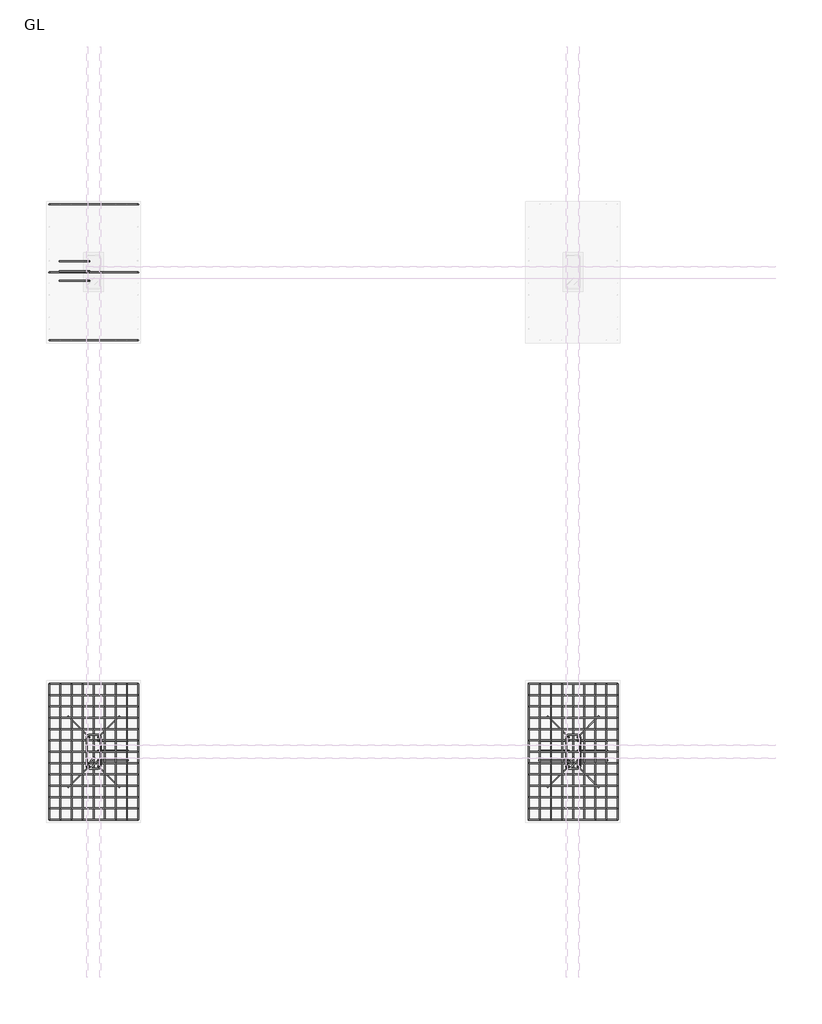
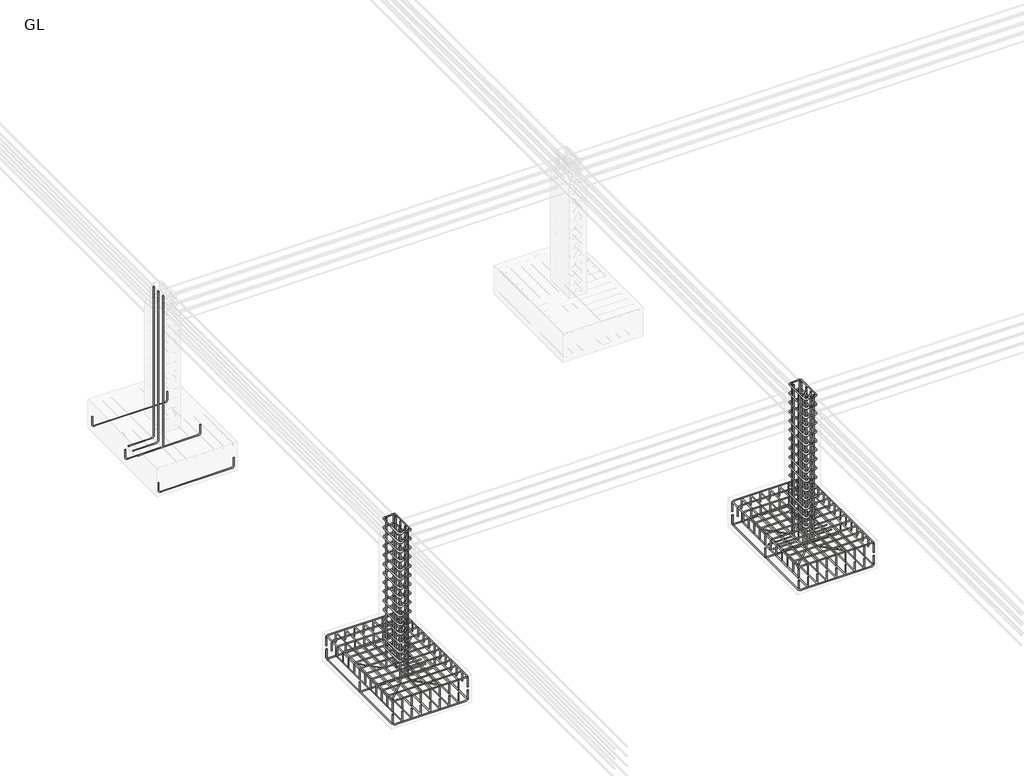
# One storey, part 4 of 16: 23 reinforcing bars.
"""IFC4 building model written with IfcOpenShell, lengths in millimetres."""

from ifc_helpers import new_model, si_unit, point, frame, origin, place, context, project, spatial, polyline, circle_curve, trimmed, segment, composite_curve, source, transform, mapped, element, save
from ifc_brep_helpers import swept_disk

model = new_model("IFC4")

# Units and contexts
model_context = context("Model", 3, world=origin())
ifc_project = project(units=[si_unit("LENGTHUNIT", "METRE", prefix="MILLI")], contexts=[model_context])

# Site, building, storey
site = spatial("IfcSite", under=ifc_project)
building = spatial("IfcBuilding", under=site)
storey = spatial("IfcBuildingStorey", under=building, Name="GL", Elevation=-1829.0)

# Reinforcing bars
placement = place(None, origin())
reinforcing_bar_shape = source(origin(), model_context, "Body", "SolidModel", [
    swept_disk(composite_curve([segment(polyline([(-22242.9544379, -7223.1167521, -2089.0), (-22242.9544379, -7223.1167521, -2213.0)]), True, "CONTINUOUS"), segment(trimmed(circle_curve(frame((-22272.9544379, -7223.1167521, -2213.0), z_axis=(0.0, 1.0, 0.0), x_axis=(30.0, 0.0, 0.0)), 30.0), [point((-22242.9544379, -7223.1167521, -2213.0))], [point((-22272.9544379, -7223.1167521, -2243.0))], True, "CARTESIAN"), True, "CONTINUOUS"), segment(polyline([(-22272.9544379, -7223.1167521, -2243.0), (-23340.9544379, -7223.1167521, -2243.0)]), True, "CONTINUOUS"), segment(trimmed(circle_curve(frame((-23340.9544379, -7223.1167521, -2213.0), z_axis=(0.0, 1.0, 0.0), x_axis=(0.0, 0.0, -30.0)), 30.0), [point((-23340.9544379, -7223.1167521, -2243.0))], [point((-23370.9544379, -7223.1167521, -2213.0))], True, "CARTESIAN"), True, "CONTINUOUS"), segment(polyline([(-23370.9544379, -7223.1167521, -2213.0), (-23370.9544379, -7223.1167521, -2089.0)]), True, "CONTINUOUS")], self_intersect=False), 6.0),
])
element("IfcReinforcingBar", 1, at=placement, inside=storey, context=model_context, shape_type="MappedRepresentation", body=[
    mapped(reinforcing_bar_shape, transform((0.0, 0.0, 0.0), x_axis=(1.0, 0.0, 0.0), y_axis=(0.0, 1.0, 0.0), z_axis=(0.0, 0.0, 1.0))),
    mapped(reinforcing_bar_shape, transform((0.0, -864.0, 0.0), x_axis=(1.0, 0.0, 0.0), y_axis=(0.0, 1.0, 0.0), z_axis=(0.0, 0.0, 1.0))),
    mapped(reinforcing_bar_shape, transform((0.0, -1728.0, 0.0), x_axis=(1.0, 0.0, 0.0), y_axis=(0.0, 1.0, 0.0), z_axis=(0.0, 0.0, 1.0))),
])
reinforcing_bar_2_shape = source(origin(), model_context, "Body", "SolidModel", [
    swept_disk(composite_curve([segment(polyline([(-16146.9544379, -13319.1167521, -2089.0), (-16146.9544379, -13319.1167521, -2213.0)]), True, "CONTINUOUS"), segment(trimmed(circle_curve(frame((-16176.9544379, -13319.1167521, -2213.0), z_axis=(0.0, 1.0, 0.0), x_axis=(30.0, 0.0, 0.0)), 30.0), [point((-16146.9544379, -13319.1167521, -2213.0))], [point((-16176.9544379, -13319.1167521, -2243.0))], True, "CARTESIAN"), True, "CONTINUOUS"), segment(polyline([(-16176.9544379, -13319.1167521, -2243.0), (-17244.9544379, -13319.1167521, -2243.0)]), True, "CONTINUOUS"), segment(trimmed(circle_curve(frame((-17244.9544379, -13319.1167521, -2213.0), z_axis=(0.0, 1.0, 0.0), x_axis=(0.0, 0.0, -30.0)), 30.0), [point((-17244.9544379, -13319.1167521, -2243.0))], [point((-17274.9544379, -13319.1167521, -2213.0))], True, "CARTESIAN"), True, "CONTINUOUS"), segment(polyline([(-17274.9544379, -13319.1167521, -2213.0), (-17274.9544379, -13319.1167521, -2089.0)]), True, "CONTINUOUS")], self_intersect=False), 6.0),
])
element("IfcReinforcingBar", 2, at=placement, inside=storey, context=model_context, shape_type="MappedRepresentation", body=[
    mapped(reinforcing_bar_2_shape, transform((0.0, 0.0, 0.0), x_axis=(1.0, 0.0, 0.0), y_axis=(0.0, 1.0, 0.0), z_axis=(0.0, 0.0, 1.0))),
    mapped(reinforcing_bar_2_shape, transform((0.0, -864.0, 0.0), x_axis=(1.0, 0.0, 0.0), y_axis=(0.0, 1.0, 0.0), z_axis=(0.0, 0.0, 1.0))),
    mapped(reinforcing_bar_2_shape, transform((0.0, -1728.0, 0.0), x_axis=(1.0, 0.0, 0.0), y_axis=(0.0, 1.0, 0.0), z_axis=(0.0, 0.0, 1.0))),
])
reinforcing_bar_3_shape = source(origin(), model_context, "Body", "SolidModel", [
    swept_disk(composite_curve([segment(polyline([(-17274.9544379, -13319.1167521, -2022.436678), (-17274.9544379, -13319.1167521, -1898.436678)]), True, "CONTINUOUS"), segment(trimmed(circle_curve(frame((-17244.9544379, -13319.1167521, -1898.436678), z_axis=(0.0, 1.0, 0.0), x_axis=(-30.0, 0.0, 0.0)), 30.0), [point((-17274.9544379, -13319.1167521, -1898.436678))], [point((-17244.9544379, -13319.1167521, -1868.436678))], True, "CARTESIAN"), True, "CONTINUOUS"), segment(polyline([(-17244.9544379, -13319.1167521, -1868.436678), (-16176.9544379, -13319.1167521, -1868.436678)]), True, "CONTINUOUS"), segment(trimmed(circle_curve(frame((-16176.9544379, -13319.1167521, -1898.436678), z_axis=(0.0, 1.0, 0.0), x_axis=(0.0, 0.0, 30.0)), 30.0), [point((-16176.9544379, -13319.1167521, -1868.436678))], [point((-16146.9544379, -13319.1167521, -1898.436678))], True, "CARTESIAN"), True, "CONTINUOUS"), segment(polyline([(-16146.9544379, -13319.1167521, -1898.436678), (-16146.9544379, -13319.1167521, -2022.436678)]), True, "CONTINUOUS")], self_intersect=False), 6.0),
])
element("IfcReinforcingBar", 3, at=placement, inside=storey, context=model_context, shape_type="MappedRepresentation", body=[
    mapped(reinforcing_bar_3_shape, transform((0.0, 0.0, 0.0), x_axis=(1.0, 0.0, 0.0), y_axis=(0.0, 1.0, 0.0), z_axis=(0.0, 0.0, 1.0))),
    mapped(reinforcing_bar_3_shape, transform((0.0, -144.0, 0.0), x_axis=(1.0, 0.0, 0.0), y_axis=(0.0, 1.0, 0.0), z_axis=(0.0, 0.0, 1.0))),
    mapped(reinforcing_bar_3_shape, transform((0.0, -288.0, 0.0), x_axis=(1.0, 0.0, 0.0), y_axis=(0.0, 1.0, 0.0), z_axis=(0.0, 0.0, 1.0))),
    mapped(reinforcing_bar_3_shape, transform((0.0, -432.0, 0.0), x_axis=(1.0, 0.0, 0.0), y_axis=(0.0, 1.0, 0.0), z_axis=(0.0, 0.0, 1.0))),
    mapped(reinforcing_bar_3_shape, transform((0.0, -576.0, 0.0), x_axis=(1.0, 0.0, 0.0), y_axis=(0.0, 1.0, 0.0), z_axis=(0.0, 0.0, 1.0))),
    mapped(reinforcing_bar_3_shape, transform((0.0, -720.0, 0.0), x_axis=(1.0, 0.0, 0.0), y_axis=(0.0, 1.0, 0.0), z_axis=(0.0, 0.0, 1.0))),
    mapped(reinforcing_bar_3_shape, transform((0.0, -864.0, 0.0), x_axis=(1.0, 0.0, 0.0), y_axis=(0.0, 1.0, 0.0), z_axis=(0.0, 0.0, 1.0))),
    mapped(reinforcing_bar_3_shape, transform((0.0, -1008.0, 0.0), x_axis=(1.0, 0.0, 0.0), y_axis=(0.0, 1.0, 0.0), z_axis=(0.0, 0.0, 1.0))),
    mapped(reinforcing_bar_3_shape, transform((0.0, -1152.0, 0.0), x_axis=(1.0, 0.0, 0.0), y_axis=(0.0, 1.0, 0.0), z_axis=(0.0, 0.0, 1.0))),
    mapped(reinforcing_bar_3_shape, transform((0.0, -1296.0, 0.0), x_axis=(1.0, 0.0, 0.0), y_axis=(0.0, 1.0, 0.0), z_axis=(0.0, 0.0, 1.0))),
    mapped(reinforcing_bar_3_shape, transform((0.0, -1440.0, 0.0), x_axis=(1.0, 0.0, 0.0), y_axis=(0.0, 1.0, 0.0), z_axis=(0.0, 0.0, 1.0))),
    mapped(reinforcing_bar_3_shape, transform((0.0, -1584.0, 0.0), x_axis=(1.0, 0.0, 0.0), y_axis=(0.0, 1.0, 0.0), z_axis=(0.0, 0.0, 1.0))),
    mapped(reinforcing_bar_3_shape, transform((0.0, -1728.0, 0.0), x_axis=(1.0, 0.0, 0.0), y_axis=(0.0, 1.0, 0.0), z_axis=(0.0, 0.0, 1.0))),
])
reinforcing_bar_4_shape = source(origin(), model_context, "Body", "SolidModel", [
    swept_disk(composite_curve([segment(polyline([(-17274.9544379, -15047.1167521, -2027.5081232), (-17274.9544379, -15047.1167521, -1903.5081232)]), True, "CONTINUOUS"), segment(trimmed(circle_curve(frame((-17274.9544379, -15017.1167521, -1903.5081232), z_axis=(-1.0, 0.0, 0.0), x_axis=(0.0, -30.0, 0.0)), 30.0), [point((-17274.9544379, -15047.1167521, -1903.5081232))], [point((-17274.9544379, -15017.1167521, -1873.5081232))], True, "CARTESIAN"), True, "CONTINUOUS"), segment(polyline([(-17274.9544379, -15017.1167521, -1873.5081232), (-17274.9544379, -13349.1167521, -1873.5081232)]), True, "CONTINUOUS"), segment(trimmed(circle_curve(frame((-17274.9544379, -13349.1167521, -1903.5081232), z_axis=(-1.0, 0.0, 0.0), x_axis=(0.0, 0.0, 30.0)), 30.0), [point((-17274.9544379, -13349.1167521, -1873.5081232))], [point((-17274.9544379, -13319.1167521, -1903.5081232))], True, "CARTESIAN"), True, "CONTINUOUS"), segment(polyline([(-17274.9544379, -13319.1167521, -1903.5081232), (-17274.9544379, -13319.1167521, -2027.5081232)]), True, "CONTINUOUS")], self_intersect=False), 6.0),
])
element("IfcReinforcingBar", 4, at=placement, inside=storey, context=model_context, shape_type="MappedRepresentation", body=[
    mapped(reinforcing_bar_4_shape, transform((0.0, 0.0, 0.0), x_axis=(1.0, 0.0, 0.0), y_axis=(0.0, 1.0, 0.0), z_axis=(0.0, 0.0, 1.0))),
    mapped(reinforcing_bar_4_shape, transform((141.0, 0.0, 0.0), x_axis=(1.0, 0.0, 0.0), y_axis=(0.0, 1.0, 0.0), z_axis=(0.0, 0.0, 1.0))),
    mapped(reinforcing_bar_4_shape, transform((282.0, 0.0, 0.0), x_axis=(1.0, 0.0, 0.0), y_axis=(0.0, 1.0, 0.0), z_axis=(0.0, 0.0, 1.0))),
    mapped(reinforcing_bar_4_shape, transform((423.0, 0.0, 0.0), x_axis=(1.0, 0.0, 0.0), y_axis=(0.0, 1.0, 0.0), z_axis=(0.0, 0.0, 1.0))),
    mapped(reinforcing_bar_4_shape, transform((564.0, 0.0, 0.0), x_axis=(1.0, 0.0, 0.0), y_axis=(0.0, 1.0, 0.0), z_axis=(0.0, 0.0, 1.0))),
    mapped(reinforcing_bar_4_shape, transform((705.0, 0.0, 0.0), x_axis=(1.0, 0.0, 0.0), y_axis=(0.0, 1.0, 0.0), z_axis=(0.0, 0.0, 1.0))),
    mapped(reinforcing_bar_4_shape, transform((846.0, 0.0, 0.0), x_axis=(1.0, 0.0, 0.0), y_axis=(0.0, 1.0, 0.0), z_axis=(0.0, 0.0, 1.0))),
    mapped(reinforcing_bar_4_shape, transform((987.0, 0.0, 0.0), x_axis=(1.0, 0.0, 0.0), y_axis=(0.0, 1.0, 0.0), z_axis=(0.0, 0.0, 1.0))),
    mapped(reinforcing_bar_4_shape, transform((1128.0, 0.0, 0.0), x_axis=(1.0, 0.0, 0.0), y_axis=(0.0, 1.0, 0.0), z_axis=(0.0, 0.0, 1.0))),
])
reinforcing_bar_5_shape = source(origin(), model_context, "Body", "SolidModel", [
    swept_disk(composite_curve([segment(polyline([(-16146.9544379, -15047.1167521, -2080.6239909), (-16146.9544379, -15047.1167521, -2204.6239909)]), True, "CONTINUOUS"), segment(trimmed(circle_curve(frame((-16146.9544379, -15017.1167521, -2204.6239909), z_axis=(1.0, 0.0, 0.0), x_axis=(0.0, -30.0, 0.0)), 30.0), [point((-16146.9544379, -15047.1167521, -2204.6239909))], [point((-16146.9544379, -15017.1167521, -2234.6239909))], True, "CARTESIAN"), True, "CONTINUOUS"), segment(polyline([(-16146.9544379, -15017.1167521, -2234.6239909), (-16146.9544379, -13362.1421892, -2234.6239909)]), True, "CONTINUOUS"), segment(trimmed(circle_curve(frame((-16146.9544379, -13362.1421892, -2204.6239909), z_axis=(1.0, 0.0, 0.0), x_axis=(0.0, 0.0, -30.0)), 30.0), [point((-16146.9544379, -13362.1421892, -2234.6239909))], [point((-16146.9544379, -13332.1421892, -2204.6239909))], True, "CARTESIAN"), True, "CONTINUOUS"), segment(polyline([(-16146.9544379, -13332.1421892, -2204.6239909), (-16146.9544379, -13332.1421892, -2080.6239909)]), True, "CONTINUOUS")], self_intersect=False), 6.0),
])
element("IfcReinforcingBar", 5, at=placement, inside=storey, context=model_context, shape_type="MappedRepresentation", body=[
    mapped(reinforcing_bar_5_shape, transform((0.0, 0.0, 0.0), x_axis=(1.0, 0.0, 0.0), y_axis=(0.0, 1.0, 0.0), z_axis=(0.0, 0.0, 1.0))),
    mapped(reinforcing_bar_5_shape, transform((-141.0, 0.0, 0.0), x_axis=(1.0, 0.0, 0.0), y_axis=(0.0, 1.0, 0.0), z_axis=(0.0, 0.0, 1.0))),
    mapped(reinforcing_bar_5_shape, transform((-282.0, 0.0, 0.0), x_axis=(1.0, 0.0, 0.0), y_axis=(0.0, 1.0, 0.0), z_axis=(0.0, 0.0, 1.0))),
    mapped(reinforcing_bar_5_shape, transform((-423.0, 0.0, 0.0), x_axis=(1.0, 0.0, 0.0), y_axis=(0.0, 1.0, 0.0), z_axis=(0.0, 0.0, 1.0))),
    mapped(reinforcing_bar_5_shape, transform((-564.0, 0.0, 0.0), x_axis=(1.0, 0.0, 0.0), y_axis=(0.0, 1.0, 0.0), z_axis=(0.0, 0.0, 1.0))),
    mapped(reinforcing_bar_5_shape, transform((-705.0, 0.0, 0.0), x_axis=(1.0, 0.0, 0.0), y_axis=(0.0, 1.0, 0.0), z_axis=(0.0, 0.0, 1.0))),
    mapped(reinforcing_bar_5_shape, transform((-846.0, 0.0, 0.0), x_axis=(1.0, 0.0, 0.0), y_axis=(0.0, 1.0, 0.0), z_axis=(0.0, 0.0, 1.0))),
    mapped(reinforcing_bar_5_shape, transform((-987.0, 0.0, 0.0), x_axis=(1.0, 0.0, 0.0), y_axis=(0.0, 1.0, 0.0), z_axis=(0.0, 0.0, 1.0))),
    mapped(reinforcing_bar_5_shape, transform((-1128.0, 0.0, 0.0), x_axis=(1.0, 0.0, 0.0), y_axis=(0.0, 1.0, 0.0), z_axis=(0.0, 0.0, 1.0))),
])
reinforcing_bar_6_shape = source(origin(), model_context, "Body", "SolidModel", [
    swept_disk(composite_curve([segment(polyline([(-22242.9544379, -13319.1167521, -2089.0), (-22242.9544379, -13319.1167521, -2213.0)]), True, "CONTINUOUS"), segment(trimmed(circle_curve(frame((-22272.9544379, -13319.1167521, -2213.0), z_axis=(0.0, 1.0, 0.0), x_axis=(30.0, 0.0, 0.0)), 30.0), [point((-22242.9544379, -13319.1167521, -2213.0))], [point((-22272.9544379, -13319.1167521, -2243.0))], True, "CARTESIAN"), True, "CONTINUOUS"), segment(polyline([(-22272.9544379, -13319.1167521, -2243.0), (-23340.9544379, -13319.1167521, -2243.0)]), True, "CONTINUOUS"), segment(trimmed(circle_curve(frame((-23340.9544379, -13319.1167521, -2213.0), z_axis=(0.0, 1.0, 0.0), x_axis=(0.0, 0.0, -30.0)), 30.0), [point((-23340.9544379, -13319.1167521, -2243.0))], [point((-23370.9544379, -13319.1167521, -2213.0))], True, "CARTESIAN"), True, "CONTINUOUS"), segment(polyline([(-23370.9544379, -13319.1167521, -2213.0), (-23370.9544379, -13319.1167521, -2089.0)]), True, "CONTINUOUS")], self_intersect=False), 6.0),
])
element("IfcReinforcingBar", 6, at=placement, inside=storey, context=model_context, shape_type="MappedRepresentation", body=[
    mapped(reinforcing_bar_6_shape, transform((0.0, 0.0, 0.0), x_axis=(1.0, 0.0, 0.0), y_axis=(0.0, 1.0, 0.0), z_axis=(0.0, 0.0, 1.0))),
    mapped(reinforcing_bar_6_shape, transform((0.0, -864.0, 0.0), x_axis=(1.0, 0.0, 0.0), y_axis=(0.0, 1.0, 0.0), z_axis=(0.0, 0.0, 1.0))),
    mapped(reinforcing_bar_6_shape, transform((0.0, -1728.0, 0.0), x_axis=(1.0, 0.0, 0.0), y_axis=(0.0, 1.0, 0.0), z_axis=(0.0, 0.0, 1.0))),
])
reinforcing_bar_7_shape = source(origin(), model_context, "Body", "SolidModel", [
    swept_disk(composite_curve([segment(polyline([(-23370.9544379, -13319.1167521, -2022.436678), (-23370.9544379, -13319.1167521, -1898.436678)]), True, "CONTINUOUS"), segment(trimmed(circle_curve(frame((-23340.9544379, -13319.1167521, -1898.436678), z_axis=(0.0, 1.0, 0.0), x_axis=(-30.0, 0.0, 0.0)), 30.0), [point((-23370.9544379, -13319.1167521, -1898.436678))], [point((-23340.9544379, -13319.1167521, -1868.436678))], True, "CARTESIAN"), True, "CONTINUOUS"), segment(polyline([(-23340.9544379, -13319.1167521, -1868.436678), (-22272.9544379, -13319.1167521, -1868.436678)]), True, "CONTINUOUS"), segment(trimmed(circle_curve(frame((-22272.9544379, -13319.1167521, -1898.436678), z_axis=(0.0, 1.0, 0.0), x_axis=(0.0, 0.0, 30.0)), 30.0), [point((-22272.9544379, -13319.1167521, -1868.436678))], [point((-22242.9544379, -13319.1167521, -1898.436678))], True, "CARTESIAN"), True, "CONTINUOUS"), segment(polyline([(-22242.9544379, -13319.1167521, -1898.436678), (-22242.9544379, -13319.1167521, -2022.436678)]), True, "CONTINUOUS")], self_intersect=False), 6.0),
])
element("IfcReinforcingBar", 7, at=placement, inside=storey, context=model_context, shape_type="MappedRepresentation", body=[
    mapped(reinforcing_bar_7_shape, transform((0.0, 0.0, 0.0), x_axis=(1.0, 0.0, 0.0), y_axis=(0.0, 1.0, 0.0), z_axis=(0.0, 0.0, 1.0))),
    mapped(reinforcing_bar_7_shape, transform((0.0, -144.0, 0.0), x_axis=(1.0, 0.0, 0.0), y_axis=(0.0, 1.0, 0.0), z_axis=(0.0, 0.0, 1.0))),
    mapped(reinforcing_bar_7_shape, transform((0.0, -288.0, 0.0), x_axis=(1.0, 0.0, 0.0), y_axis=(0.0, 1.0, 0.0), z_axis=(0.0, 0.0, 1.0))),
    mapped(reinforcing_bar_7_shape, transform((0.0, -432.0, 0.0), x_axis=(1.0, 0.0, 0.0), y_axis=(0.0, 1.0, 0.0), z_axis=(0.0, 0.0, 1.0))),
    mapped(reinforcing_bar_7_shape, transform((0.0, -576.0, 0.0), x_axis=(1.0, 0.0, 0.0), y_axis=(0.0, 1.0, 0.0), z_axis=(0.0, 0.0, 1.0))),
    mapped(reinforcing_bar_7_shape, transform((0.0, -720.0, 0.0), x_axis=(1.0, 0.0, 0.0), y_axis=(0.0, 1.0, 0.0), z_axis=(0.0, 0.0, 1.0))),
    mapped(reinforcing_bar_7_shape, transform((0.0, -864.0, 0.0), x_axis=(1.0, 0.0, 0.0), y_axis=(0.0, 1.0, 0.0), z_axis=(0.0, 0.0, 1.0))),
    mapped(reinforcing_bar_7_shape, transform((0.0, -1008.0, 0.0), x_axis=(1.0, 0.0, 0.0), y_axis=(0.0, 1.0, 0.0), z_axis=(0.0, 0.0, 1.0))),
    mapped(reinforcing_bar_7_shape, transform((0.0, -1152.0, 0.0), x_axis=(1.0, 0.0, 0.0), y_axis=(0.0, 1.0, 0.0), z_axis=(0.0, 0.0, 1.0))),
    mapped(reinforcing_bar_7_shape, transform((0.0, -1296.0, 0.0), x_axis=(1.0, 0.0, 0.0), y_axis=(0.0, 1.0, 0.0), z_axis=(0.0, 0.0, 1.0))),
    mapped(reinforcing_bar_7_shape, transform((0.0, -1440.0, 0.0), x_axis=(1.0, 0.0, 0.0), y_axis=(0.0, 1.0, 0.0), z_axis=(0.0, 0.0, 1.0))),
    mapped(reinforcing_bar_7_shape, transform((0.0, -1584.0, 0.0), x_axis=(1.0, 0.0, 0.0), y_axis=(0.0, 1.0, 0.0), z_axis=(0.0, 0.0, 1.0))),
    mapped(reinforcing_bar_7_shape, transform((0.0, -1728.0, 0.0), x_axis=(1.0, 0.0, 0.0), y_axis=(0.0, 1.0, 0.0), z_axis=(0.0, 0.0, 1.0))),
])
reinforcing_bar_8_shape = source(origin(), model_context, "Body", "SolidModel", [
    swept_disk(composite_curve([segment(polyline([(-23370.9544379, -15047.1167521, -2027.5081232), (-23370.9544379, -15047.1167521, -1903.5081232)]), True, "CONTINUOUS"), segment(trimmed(circle_curve(frame((-23370.9544379, -15017.1167521, -1903.5081232), z_axis=(-1.0, 0.0, 0.0), x_axis=(0.0, -30.0, 0.0)), 30.0), [point((-23370.9544379, -15047.1167521, -1903.5081232))], [point((-23370.9544379, -15017.1167521, -1873.5081232))], True, "CARTESIAN"), True, "CONTINUOUS"), segment(polyline([(-23370.9544379, -15017.1167521, -1873.5081232), (-23370.9544379, -13349.1167521, -1873.5081232)]), True, "CONTINUOUS"), segment(trimmed(circle_curve(frame((-23370.9544379, -13349.1167521, -1903.5081232), z_axis=(-1.0, 0.0, 0.0), x_axis=(0.0, 0.0, 30.0)), 30.0), [point((-23370.9544379, -13349.1167521, -1873.5081232))], [point((-23370.9544379, -13319.1167521, -1903.5081232))], True, "CARTESIAN"), True, "CONTINUOUS"), segment(polyline([(-23370.9544379, -13319.1167521, -1903.5081232), (-23370.9544379, -13319.1167521, -2027.5081232)]), True, "CONTINUOUS")], self_intersect=False), 6.0),
])
element("IfcReinforcingBar", 8, at=placement, inside=storey, context=model_context, shape_type="MappedRepresentation", body=[
    mapped(reinforcing_bar_8_shape, transform((0.0, 0.0, 0.0), x_axis=(1.0, 0.0, 0.0), y_axis=(0.0, 1.0, 0.0), z_axis=(0.0, 0.0, 1.0))),
    mapped(reinforcing_bar_8_shape, transform((141.0, 0.0, 0.0), x_axis=(1.0, 0.0, 0.0), y_axis=(0.0, 1.0, 0.0), z_axis=(0.0, 0.0, 1.0))),
    mapped(reinforcing_bar_8_shape, transform((282.0, 0.0, 0.0), x_axis=(1.0, 0.0, 0.0), y_axis=(0.0, 1.0, 0.0), z_axis=(0.0, 0.0, 1.0))),
    mapped(reinforcing_bar_8_shape, transform((423.0, 0.0, 0.0), x_axis=(1.0, 0.0, 0.0), y_axis=(0.0, 1.0, 0.0), z_axis=(0.0, 0.0, 1.0))),
    mapped(reinforcing_bar_8_shape, transform((564.0, 0.0, 0.0), x_axis=(1.0, 0.0, 0.0), y_axis=(0.0, 1.0, 0.0), z_axis=(0.0, 0.0, 1.0))),
    mapped(reinforcing_bar_8_shape, transform((705.0, 0.0, 0.0), x_axis=(1.0, 0.0, 0.0), y_axis=(0.0, 1.0, 0.0), z_axis=(0.0, 0.0, 1.0))),
    mapped(reinforcing_bar_8_shape, transform((846.0, 0.0, 0.0), x_axis=(1.0, 0.0, 0.0), y_axis=(0.0, 1.0, 0.0), z_axis=(0.0, 0.0, 1.0))),
    mapped(reinforcing_bar_8_shape, transform((987.0, 0.0, 0.0), x_axis=(1.0, 0.0, 0.0), y_axis=(0.0, 1.0, 0.0), z_axis=(0.0, 0.0, 1.0))),
    mapped(reinforcing_bar_8_shape, transform((1128.0, 0.0, 0.0), x_axis=(1.0, 0.0, 0.0), y_axis=(0.0, 1.0, 0.0), z_axis=(0.0, 0.0, 1.0))),
])
reinforcing_bar_9_shape = source(origin(), model_context, "Body", "SolidModel", [
    swept_disk(composite_curve([segment(polyline([(-22242.9544379, -15047.1167521, -2080.6239909), (-22242.9544379, -15047.1167521, -2204.6239909)]), True, "CONTINUOUS"), segment(trimmed(circle_curve(frame((-22242.9544379, -15017.1167521, -2204.6239909), z_axis=(1.0, 0.0, 0.0), x_axis=(0.0, -30.0, 0.0)), 30.0), [point((-22242.9544379, -15047.1167521, -2204.6239909))], [point((-22242.9544379, -15017.1167521, -2234.6239909))], True, "CARTESIAN"), True, "CONTINUOUS"), segment(polyline([(-22242.9544379, -15017.1167521, -2234.6239909), (-22242.9544379, -13362.1421892, -2234.6239909)]), True, "CONTINUOUS"), segment(trimmed(circle_curve(frame((-22242.9544379, -13362.1421892, -2204.6239909), z_axis=(1.0, 0.0, 0.0), x_axis=(0.0, 0.0, -30.0)), 30.0), [point((-22242.9544379, -13362.1421892, -2234.6239909))], [point((-22242.9544379, -13332.1421892, -2204.6239909))], True, "CARTESIAN"), True, "CONTINUOUS"), segment(polyline([(-22242.9544379, -13332.1421892, -2204.6239909), (-22242.9544379, -13332.1421892, -2080.6239909)]), True, "CONTINUOUS")], self_intersect=False), 6.0),
])
element("IfcReinforcingBar", 9, at=placement, inside=storey, context=model_context, shape_type="MappedRepresentation", body=[
    mapped(reinforcing_bar_9_shape, transform((0.0, 0.0, 0.0), x_axis=(1.0, 0.0, 0.0), y_axis=(0.0, 1.0, 0.0), z_axis=(0.0, 0.0, 1.0))),
    mapped(reinforcing_bar_9_shape, transform((-141.0, 0.0, 0.0), x_axis=(1.0, 0.0, 0.0), y_axis=(0.0, 1.0, 0.0), z_axis=(0.0, 0.0, 1.0))),
    mapped(reinforcing_bar_9_shape, transform((-282.0, 0.0, 0.0), x_axis=(1.0, 0.0, 0.0), y_axis=(0.0, 1.0, 0.0), z_axis=(0.0, 0.0, 1.0))),
    mapped(reinforcing_bar_9_shape, transform((-423.0, 0.0, 0.0), x_axis=(1.0, 0.0, 0.0), y_axis=(0.0, 1.0, 0.0), z_axis=(0.0, 0.0, 1.0))),
    mapped(reinforcing_bar_9_shape, transform((-564.0, 0.0, 0.0), x_axis=(1.0, 0.0, 0.0), y_axis=(0.0, 1.0, 0.0), z_axis=(0.0, 0.0, 1.0))),
    mapped(reinforcing_bar_9_shape, transform((-705.0, 0.0, 0.0), x_axis=(1.0, 0.0, 0.0), y_axis=(0.0, 1.0, 0.0), z_axis=(0.0, 0.0, 1.0))),
    mapped(reinforcing_bar_9_shape, transform((-846.0, 0.0, 0.0), x_axis=(1.0, 0.0, 0.0), y_axis=(0.0, 1.0, 0.0), z_axis=(0.0, 0.0, 1.0))),
    mapped(reinforcing_bar_9_shape, transform((-987.0, 0.0, 0.0), x_axis=(1.0, 0.0, 0.0), y_axis=(0.0, 1.0, 0.0), z_axis=(0.0, 0.0, 1.0))),
    mapped(reinforcing_bar_9_shape, transform((-1128.0, 0.0, 0.0), x_axis=(1.0, 0.0, 0.0), y_axis=(0.0, 1.0, 0.0), z_axis=(0.0, 0.0, 1.0))),
])
reinforcing_bar_10_shape = source(origin(), model_context, "Body", "SolidModel", [
    swept_disk(composite_curve([segment(polyline([(-22864.0642232, -8194.9117405, 241.0), (-22864.0642232, -8194.9117405, -2129.0)]), True, "CONTINUOUS"), segment(trimmed(circle_curve(frame((-22894.0642232, -8194.9117405, -2129.0), z_axis=(0.0, 1.0, 0.0), x_axis=(30.0, 0.0, 0.0)), 30.0), [point((-22864.0642232, -8194.9117405, -2129.0))], [point((-22894.0642232, -8194.9117405, -2159.0))], True, "CARTESIAN"), True, "CONTINUOUS"), segment(polyline([(-22894.0642232, -8194.9117405, -2159.0), (-23244.0642232, -8194.9117405, -2159.0)]), True, "CONTINUOUS")], self_intersect=False), 6.0),
])
element("IfcReinforcingBar", 10, at=placement, inside=storey, context=model_context, shape_type="MappedRepresentation", body=[
    mapped(reinforcing_bar_10_shape, transform((0.0, 0.0, 0.0), x_axis=(1.0, 0.0, 0.0), y_axis=(0.0, 1.0, 0.0), z_axis=(0.0, 0.0, 1.0))),
    mapped(reinforcing_bar_10_shape, transform((0.0, 123.5823926, 0.0), x_axis=(1.0, 0.0, 0.0), y_axis=(0.0, 1.0, 0.0), z_axis=(0.0, 0.0, 1.0))),
    mapped(reinforcing_bar_10_shape, transform((0.0, 247.1647853, 0.0), x_axis=(1.0, 0.0, 0.0), y_axis=(0.0, 1.0, 0.0), z_axis=(0.0, 0.0, 1.0))),
])
reinforcing_bar_11_shape = source(origin(), model_context, "Body", "SolidModel", [
    swept_disk(composite_curve([segment(polyline([(-22799.4864005, -14258.2223078, -1793.0), (-22887.1676414, -14345.9035486, -1793.0)]), True, "CONTINUOUS"), segment(trimmed(circle_curve(frame((-22865.9544379, -14367.1167521, -1793.0), z_axis=(0.0, 0.0, 1.0), x_axis=(-21.21320349999951, 21.213203500001327, 0.0)), 30.0), [point((-22887.1676414, -14345.9035486, -1793.0))], [point((-22865.9544379, -14397.1167521, -1793.0))], True, "CARTESIAN"), True, "CONTINUOUS"), segment(polyline([(-22865.9544379, -14397.1167521, -1793.0), (-22747.9544379, -14397.1167521, -1793.0)]), True, "CONTINUOUS"), segment(trimmed(circle_curve(frame((-22747.9544379, -14367.1167521, -1793.0), z_axis=(0.0, 0.0, 1.0), x_axis=(0.0, -30.0, 0.0)), 30.0), [point((-22747.9544379, -14397.1167521, -1793.0))], [point((-22717.9544379, -14367.1167521, -1793.0))], True, "CARTESIAN"), True, "CONTINUOUS"), segment(polyline([(-22717.9544379, -14367.1167521, -1793.0), (-22717.9544379, -13999.1167521, -1793.0)]), True, "CONTINUOUS"), segment(trimmed(circle_curve(frame((-22747.8864962, -13999.1167521, -1795.0178916), z_axis=(-0.06726305234213417, 0.0, 0.9977352764083365), x_axis=(29.93205830000079, 0.0, 2.0178915999999845)), 30.0), [point((-22717.9544379, -13999.1167521, -1793.0))], [point((-22747.8864962, -13969.1167521, -1795.0178916))], True, "CARTESIAN"), True, "CONTINUOUS"), segment(polyline([(-22747.8864962, -13969.1167521, -1795.0178916), (-22866.0223796, -13969.1167521, -1802.9821084)]), True, "CONTINUOUS"), segment(trimmed(circle_curve(frame((-22866.0223796, -13999.1167521, -1802.9821084), z_axis=(-0.06726305234213417, 0.0, 0.9977352764083365), x_axis=(0.0, 30.0, 0.0)), 30.0), [point((-22866.0223796, -13969.1167521, -1802.9821084))], [point((-22895.9544379, -13999.1167521, -1805.0))], True, "CARTESIAN"), True, "CONTINUOUS"), segment(polyline([(-22895.9544379, -13999.1167521, -1805.0), (-22895.9544379, -14367.1167521, -1805.0)]), True, "CONTINUOUS"), segment(trimmed(circle_curve(frame((-22865.9544379, -14367.1167521, -1805.0), z_axis=(0.0, 0.0, 1.0), x_axis=(-30.0, 0.0, 0.0)), 30.0), [point((-22895.9544379, -14367.1167521, -1805.0))], [point((-22844.7412345, -14388.3299555, -1805.0))], True, "CARTESIAN"), True, "CONTINUOUS"), segment(polyline([(-22844.7412345, -14388.3299555, -1805.0), (-22757.0599936, -14300.6487146, -1805.0)]), True, "CONTINUOUS")], self_intersect=False), 6.0),
])
element("IfcReinforcingBar", 11, at=placement, inside=storey, context=model_context, shape_type="MappedRepresentation", body=[
    mapped(reinforcing_bar_11_shape, transform((0.0, 0.0, 0.0), x_axis=(1.0, 0.0, 0.0), y_axis=(0.0, 1.0, 0.0), z_axis=(0.0, 0.0, 1.0))),
    mapped(reinforcing_bar_11_shape, transform((0.0, 0.0, 144.8571429), x_axis=(1.0, 0.0, 0.0), y_axis=(0.0, 1.0, 0.0), z_axis=(0.0, 0.0, 1.0))),
    mapped(reinforcing_bar_11_shape, transform((0.0, 0.0, 289.7142857), x_axis=(1.0, 0.0, 0.0), y_axis=(0.0, 1.0, 0.0), z_axis=(0.0, 0.0, 1.0))),
    mapped(reinforcing_bar_11_shape, transform((0.0, 0.0, 434.5714286), x_axis=(1.0, 0.0, 0.0), y_axis=(0.0, 1.0, 0.0), z_axis=(0.0, 0.0, 1.0))),
    mapped(reinforcing_bar_11_shape, transform((0.0, 0.0, 579.4285714), x_axis=(1.0, 0.0, 0.0), y_axis=(0.0, 1.0, 0.0), z_axis=(0.0, 0.0, 1.0))),
    mapped(reinforcing_bar_11_shape, transform((0.0, 0.0, 724.2857143), x_axis=(1.0, 0.0, 0.0), y_axis=(0.0, 1.0, 0.0), z_axis=(0.0, 0.0, 1.0))),
    mapped(reinforcing_bar_11_shape, transform((0.0, 0.0, 869.1428571), x_axis=(1.0, 0.0, 0.0), y_axis=(0.0, 1.0, 0.0), z_axis=(0.0, 0.0, 1.0))),
    mapped(reinforcing_bar_11_shape, transform((0.0, 0.0, 1014.0), x_axis=(1.0, 0.0, 0.0), y_axis=(0.0, 1.0, 0.0), z_axis=(0.0, 0.0, 1.0))),
    mapped(reinforcing_bar_11_shape, transform((0.0, 0.0, 1158.8571429), x_axis=(1.0, 0.0, 0.0), y_axis=(0.0, 1.0, 0.0), z_axis=(0.0, 0.0, 1.0))),
    mapped(reinforcing_bar_11_shape, transform((0.0, 0.0, 1303.7142857), x_axis=(1.0, 0.0, 0.0), y_axis=(0.0, 1.0, 0.0), z_axis=(0.0, 0.0, 1.0))),
    mapped(reinforcing_bar_11_shape, transform((0.0, 0.0, 1448.5714286), x_axis=(1.0, 0.0, 0.0), y_axis=(0.0, 1.0, 0.0), z_axis=(0.0, 0.0, 1.0))),
    mapped(reinforcing_bar_11_shape, transform((0.0, 0.0, 1593.4285714), x_axis=(1.0, 0.0, 0.0), y_axis=(0.0, 1.0, 0.0), z_axis=(0.0, 0.0, 1.0))),
    mapped(reinforcing_bar_11_shape, transform((0.0, 0.0, 1738.2857143), x_axis=(1.0, 0.0, 0.0), y_axis=(0.0, 1.0, 0.0), z_axis=(0.0, 0.0, 1.0))),
    mapped(reinforcing_bar_11_shape, transform((0.0, 0.0, 1883.1428571), x_axis=(1.0, 0.0, 0.0), y_axis=(0.0, 1.0, 0.0), z_axis=(0.0, 0.0, 1.0))),
    mapped(reinforcing_bar_11_shape, transform((0.0, 0.0, 2028.0), x_axis=(1.0, 0.0, 0.0), y_axis=(0.0, 1.0, 0.0), z_axis=(0.0, 0.0, 1.0))),
])
element("IfcReinforcingBar", 12, at=placement, inside=storey, context=model_context, shape_type="SolidModel", body=[
    swept_disk(composite_curve([segment(polyline([(-22864.0642232, -14368.0642439, 241.0), (-22864.0642232, -14368.0642439, -2129.0)]), True, "CONTINUOUS"), segment(trimmed(circle_curve(frame((-22885.2774266, -14389.2774473, -2129.0), z_axis=(-0.7071067811865187, 0.7071067811865764, 0.0), x_axis=(21.213203400002385, 21.213203400000566, 0.0)), 30.0), [point((-22864.0642232, -14368.0642439, -2129.0))], [point((-22885.2774266, -14389.2774473, -2159.0))], True, "CARTESIAN"), True, "CONTINUOUS"), segment(polyline([(-22885.2774266, -14389.2774473, -2159.0), (-23132.7648, -14636.7648207, -2159.0)]), True, "CONTINUOUS")], self_intersect=False), 6.0),
])
element("IfcReinforcingBar", 13, at=placement, inside=storey, context=model_context, shape_type="SolidModel", body=[
    swept_disk(composite_curve([segment(polyline([(-22864.0642232, -13998.1692603, 241.0), (-22864.0642232, -13998.1692603, -2129.0)]), True, "CONTINUOUS"), segment(trimmed(circle_curve(frame((-22885.2774266, -13976.9560568, -2129.0), z_axis=(0.7071067811865218, 0.7071067811865733, 0.0), x_axis=(21.213203400002385, -21.21320349999951, 0.0)), 30.0), [point((-22864.0642232, -13998.1692603, -2129.0))], [point((-22885.2774266, -13976.9560568, -2159.0))], True, "CARTESIAN"), True, "CONTINUOUS"), segment(polyline([(-22885.2774266, -13976.9560568, -2159.0), (-23132.7648, -13729.4686834, -2159.0)]), True, "CONTINUOUS")], self_intersect=False), 6.0),
])
element("IfcReinforcingBar", 14, at=placement, inside=storey, context=model_context, shape_type="SolidModel", body=[
    swept_disk(composite_curve([segment(polyline([(-22749.8446527, -14368.0642439, 241.0), (-22749.8446527, -14368.0642439, -2129.0)]), True, "CONTINUOUS"), segment(trimmed(circle_curve(frame((-22728.6314492, -14389.2774473, -2129.0), z_axis=(-0.7071067811865248, -0.7071067811865703, 0.0), x_axis=(-21.213203500003146, 21.213203400000566, 0.0)), 30.0), [point((-22749.8446527, -14368.0642439, -2129.0))], [point((-22728.6314492, -14389.2774473, -2159.0))], True, "CARTESIAN"), True, "CONTINUOUS"), segment(polyline([(-22728.6314492, -14389.2774473, -2159.0), (-22481.1440758, -14636.7648207, -2159.0)]), True, "CONTINUOUS")], self_intersect=False), 6.0),
])
element("IfcReinforcingBar", 15, at=placement, inside=storey, context=model_context, shape_type="SolidModel", body=[
    swept_disk(composite_curve([segment(polyline([(-22749.8446527, -13998.1692603, 241.0), (-22749.8446527, -13998.1692603, -2129.0)]), True, "CONTINUOUS"), segment(trimmed(circle_curve(frame((-22728.6314492, -13976.9560568, -2129.0), z_axis=(0.7071067811865157, -0.7071067811865794, 0.0), x_axis=(-21.213203500003146, -21.21320349999951, 0.0)), 30.0), [point((-22749.8446527, -13998.1692603, -2129.0))], [point((-22728.6314492, -13976.9560568, -2159.0))], True, "CARTESIAN"), True, "CONTINUOUS"), segment(polyline([(-22728.6314492, -13976.9560568, -2159.0), (-22481.1440758, -13729.4686834, -2159.0)]), True, "CONTINUOUS")], self_intersect=False), 6.0),
])
reinforcing_bar_12_shape = source(origin(), model_context, "Body", "SolidModel", [
    swept_disk(composite_curve([segment(polyline([(-22749.8446527, -14290.9117405, 241.0), (-22749.8446527, -14290.9117405, -2129.0)]), True, "CONTINUOUS"), segment(trimmed(circle_curve(frame((-22719.8446527, -14290.9117405, -2129.0), z_axis=(0.0, -1.0, 0.0), x_axis=(-30.0, 0.0, 0.0)), 30.0), [point((-22749.8446527, -14290.9117405, -2129.0))], [point((-22719.8446527, -14290.9117405, -2159.0))], True, "CARTESIAN"), True, "CONTINUOUS"), segment(polyline([(-22719.8446527, -14290.9117405, -2159.0), (-22369.8446527, -14290.9117405, -2159.0)]), True, "CONTINUOUS")], self_intersect=False), 6.0),
])
element("IfcReinforcingBar", 16, at=placement, inside=storey, context=model_context, shape_type="MappedRepresentation", body=[
    mapped(reinforcing_bar_12_shape, transform((0.0, 0.0, 0.0), x_axis=(1.0, 0.0, 0.0), y_axis=(0.0, 1.0, 0.0), z_axis=(0.0, 0.0, 1.0))),
    mapped(reinforcing_bar_12_shape, transform((0.0, 123.5823926, 0.0), x_axis=(1.0, 0.0, 0.0), y_axis=(0.0, 1.0, 0.0), z_axis=(0.0, 0.0, 1.0))),
    mapped(reinforcing_bar_12_shape, transform((0.0, 247.1647853, 0.0), x_axis=(1.0, 0.0, 0.0), y_axis=(0.0, 1.0, 0.0), z_axis=(0.0, 0.0, 1.0))),
])
reinforcing_bar_13_shape = source(origin(), model_context, "Body", "SolidModel", [
    swept_disk(composite_curve([segment(polyline([(-16703.4864005, -14258.2223078, -1793.0), (-16791.1676414, -14345.9035486, -1793.0)]), True, "CONTINUOUS"), segment(trimmed(circle_curve(frame((-16769.9544379, -14367.1167521, -1793.0), z_axis=(0.0, 0.0, 1.0), x_axis=(-21.21320349999951, 21.213203500001327, 0.0)), 30.0), [point((-16791.1676414, -14345.9035486, -1793.0))], [point((-16769.9544379, -14397.1167521, -1793.0))], True, "CARTESIAN"), True, "CONTINUOUS"), segment(polyline([(-16769.9544379, -14397.1167521, -1793.0), (-16651.9544379, -14397.1167521, -1793.0)]), True, "CONTINUOUS"), segment(trimmed(circle_curve(frame((-16651.9544379, -14367.1167521, -1793.0), z_axis=(0.0, 0.0, 1.0), x_axis=(0.0, -30.0, 0.0)), 30.0), [point((-16651.9544379, -14397.1167521, -1793.0))], [point((-16621.9544379, -14367.1167521, -1793.0))], True, "CARTESIAN"), True, "CONTINUOUS"), segment(polyline([(-16621.9544379, -14367.1167521, -1793.0), (-16621.9544379, -13999.1167521, -1793.0)]), True, "CONTINUOUS"), segment(trimmed(circle_curve(frame((-16651.8864962, -13999.1167521, -1795.0178916), z_axis=(-0.06726305234213417, 0.0, 0.9977352764083365), x_axis=(29.93205830000079, 0.0, 2.0178915999999845)), 30.0), [point((-16621.9544379, -13999.1167521, -1793.0))], [point((-16651.8864962, -13969.1167521, -1795.0178916))], True, "CARTESIAN"), True, "CONTINUOUS"), segment(polyline([(-16651.8864962, -13969.1167521, -1795.0178916), (-16770.0223796, -13969.1167521, -1802.9821084)]), True, "CONTINUOUS"), segment(trimmed(circle_curve(frame((-16770.0223796, -13999.1167521, -1802.9821084), z_axis=(-0.06726305234213417, 0.0, 0.9977352764083365), x_axis=(0.0, 30.0, 0.0)), 30.0), [point((-16770.0223796, -13969.1167521, -1802.9821084))], [point((-16799.9544379, -13999.1167521, -1805.0))], True, "CARTESIAN"), True, "CONTINUOUS"), segment(polyline([(-16799.9544379, -13999.1167521, -1805.0), (-16799.9544379, -14367.1167521, -1805.0)]), True, "CONTINUOUS"), segment(trimmed(circle_curve(frame((-16769.9544379, -14367.1167521, -1805.0), z_axis=(0.0, 0.0, 1.0), x_axis=(-30.0, 0.0, 0.0)), 30.0), [point((-16799.9544379, -14367.1167521, -1805.0))], [point((-16748.7412345, -14388.3299555, -1805.0))], True, "CARTESIAN"), True, "CONTINUOUS"), segment(polyline([(-16748.7412345, -14388.3299555, -1805.0), (-16661.0599936, -14300.6487146, -1805.0)]), True, "CONTINUOUS")], self_intersect=False), 6.0),
])
element("IfcReinforcingBar", 17, at=placement, inside=storey, context=model_context, shape_type="MappedRepresentation", body=[
    mapped(reinforcing_bar_13_shape, transform((0.0, 0.0, 0.0), x_axis=(1.0, 0.0, 0.0), y_axis=(0.0, 1.0, 0.0), z_axis=(0.0, 0.0, 1.0))),
    mapped(reinforcing_bar_13_shape, transform((0.0, 0.0, 144.8571429), x_axis=(1.0, 0.0, 0.0), y_axis=(0.0, 1.0, 0.0), z_axis=(0.0, 0.0, 1.0))),
    mapped(reinforcing_bar_13_shape, transform((0.0, 0.0, 289.7142857), x_axis=(1.0, 0.0, 0.0), y_axis=(0.0, 1.0, 0.0), z_axis=(0.0, 0.0, 1.0))),
    mapped(reinforcing_bar_13_shape, transform((0.0, 0.0, 434.5714286), x_axis=(1.0, 0.0, 0.0), y_axis=(0.0, 1.0, 0.0), z_axis=(0.0, 0.0, 1.0))),
    mapped(reinforcing_bar_13_shape, transform((0.0, 0.0, 579.4285714), x_axis=(1.0, 0.0, 0.0), y_axis=(0.0, 1.0, 0.0), z_axis=(0.0, 0.0, 1.0))),
    mapped(reinforcing_bar_13_shape, transform((0.0, 0.0, 724.2857143), x_axis=(1.0, 0.0, 0.0), y_axis=(0.0, 1.0, 0.0), z_axis=(0.0, 0.0, 1.0))),
    mapped(reinforcing_bar_13_shape, transform((0.0, 0.0, 869.1428571), x_axis=(1.0, 0.0, 0.0), y_axis=(0.0, 1.0, 0.0), z_axis=(0.0, 0.0, 1.0))),
    mapped(reinforcing_bar_13_shape, transform((0.0, 0.0, 1014.0), x_axis=(1.0, 0.0, 0.0), y_axis=(0.0, 1.0, 0.0), z_axis=(0.0, 0.0, 1.0))),
    mapped(reinforcing_bar_13_shape, transform((0.0, 0.0, 1158.8571429), x_axis=(1.0, 0.0, 0.0), y_axis=(0.0, 1.0, 0.0), z_axis=(0.0, 0.0, 1.0))),
    mapped(reinforcing_bar_13_shape, transform((0.0, 0.0, 1303.7142857), x_axis=(1.0, 0.0, 0.0), y_axis=(0.0, 1.0, 0.0), z_axis=(0.0, 0.0, 1.0))),
    mapped(reinforcing_bar_13_shape, transform((0.0, 0.0, 1448.5714286), x_axis=(1.0, 0.0, 0.0), y_axis=(0.0, 1.0, 0.0), z_axis=(0.0, 0.0, 1.0))),
    mapped(reinforcing_bar_13_shape, transform((0.0, 0.0, 1593.4285714), x_axis=(1.0, 0.0, 0.0), y_axis=(0.0, 1.0, 0.0), z_axis=(0.0, 0.0, 1.0))),
    mapped(reinforcing_bar_13_shape, transform((0.0, 0.0, 1738.2857143), x_axis=(1.0, 0.0, 0.0), y_axis=(0.0, 1.0, 0.0), z_axis=(0.0, 0.0, 1.0))),
    mapped(reinforcing_bar_13_shape, transform((0.0, 0.0, 1883.1428571), x_axis=(1.0, 0.0, 0.0), y_axis=(0.0, 1.0, 0.0), z_axis=(0.0, 0.0, 1.0))),
    mapped(reinforcing_bar_13_shape, transform((0.0, 0.0, 2028.0), x_axis=(1.0, 0.0, 0.0), y_axis=(0.0, 1.0, 0.0), z_axis=(0.0, 0.0, 1.0))),
])
element("IfcReinforcingBar", 18, at=placement, inside=storey, context=model_context, shape_type="SolidModel", body=[
    swept_disk(composite_curve([segment(polyline([(-16768.0642232, -14368.0642439, 241.0), (-16768.0642232, -14368.0642439, -2129.0)]), True, "CONTINUOUS"), segment(trimmed(circle_curve(frame((-16789.2774266, -14389.2774473, -2129.0), z_axis=(-0.7071067811865187, 0.7071067811865764, 0.0), x_axis=(21.213203400002385, 21.213203400000566, 0.0)), 30.0), [point((-16768.0642232, -14368.0642439, -2129.0))], [point((-16789.2774266, -14389.2774473, -2159.0))], True, "CARTESIAN"), True, "CONTINUOUS"), segment(polyline([(-16789.2774266, -14389.2774473, -2159.0), (-17036.7648, -14636.7648207, -2159.0)]), True, "CONTINUOUS")], self_intersect=False), 6.0),
])
element("IfcReinforcingBar", 19, at=placement, inside=storey, context=model_context, shape_type="SolidModel", body=[
    swept_disk(composite_curve([segment(polyline([(-16768.0642232, -13998.1692603, 241.0), (-16768.0642232, -13998.1692603, -2129.0)]), True, "CONTINUOUS"), segment(trimmed(circle_curve(frame((-16789.2774266, -13976.9560568, -2129.0), z_axis=(0.7071067811865218, 0.7071067811865733, 0.0), x_axis=(21.213203400002385, -21.21320349999951, 0.0)), 30.0), [point((-16768.0642232, -13998.1692603, -2129.0))], [point((-16789.2774266, -13976.9560568, -2159.0))], True, "CARTESIAN"), True, "CONTINUOUS"), segment(polyline([(-16789.2774266, -13976.9560568, -2159.0), (-17036.7648, -13729.4686834, -2159.0)]), True, "CONTINUOUS")], self_intersect=False), 6.0),
])
element("IfcReinforcingBar", 20, at=placement, inside=storey, context=model_context, shape_type="SolidModel", body=[
    swept_disk(composite_curve([segment(polyline([(-16653.8446527, -14368.0642439, 241.0), (-16653.8446527, -14368.0642439, -2129.0)]), True, "CONTINUOUS"), segment(trimmed(circle_curve(frame((-16632.6314492, -14389.2774473, -2129.0), z_axis=(-0.7071067811865248, -0.7071067811865703, 0.0), x_axis=(-21.213203500003146, 21.213203400000566, 0.0)), 30.0), [point((-16653.8446527, -14368.0642439, -2129.0))], [point((-16632.6314492, -14389.2774473, -2159.0))], True, "CARTESIAN"), True, "CONTINUOUS"), segment(polyline([(-16632.6314492, -14389.2774473, -2159.0), (-16385.1440758, -14636.7648207, -2159.0)]), True, "CONTINUOUS")], self_intersect=False), 6.0),
])
element("IfcReinforcingBar", 21, at=placement, inside=storey, context=model_context, shape_type="SolidModel", body=[
    swept_disk(composite_curve([segment(polyline([(-16653.8446527, -13998.1692603, 241.0), (-16653.8446527, -13998.1692603, -2129.0)]), True, "CONTINUOUS"), segment(trimmed(circle_curve(frame((-16632.6314492, -13976.9560568, -2129.0), z_axis=(0.7071067811865157, -0.7071067811865794, 0.0), x_axis=(-21.213203500003146, -21.21320349999951, 0.0)), 30.0), [point((-16653.8446527, -13998.1692603, -2129.0))], [point((-16632.6314492, -13976.9560568, -2159.0))], True, "CARTESIAN"), True, "CONTINUOUS"), segment(polyline([(-16632.6314492, -13976.9560568, -2159.0), (-16385.1440758, -13729.4686834, -2159.0)]), True, "CONTINUOUS")], self_intersect=False), 6.0),
])
reinforcing_bar_14_shape = source(origin(), model_context, "Body", "SolidModel", [
    swept_disk(composite_curve([segment(polyline([(-16768.0642232, -14290.9117405, 241.0), (-16768.0642232, -14290.9117405, -2129.0)]), True, "CONTINUOUS"), segment(trimmed(circle_curve(frame((-16798.0642232, -14290.9117405, -2129.0), z_axis=(0.0, 1.0, 0.0), x_axis=(30.0, 0.0, 0.0)), 30.0), [point((-16768.0642232, -14290.9117405, -2129.0))], [point((-16798.0642232, -14290.9117405, -2159.0))], True, "CARTESIAN"), True, "CONTINUOUS"), segment(polyline([(-16798.0642232, -14290.9117405, -2159.0), (-17148.0642232, -14290.9117405, -2159.0)]), True, "CONTINUOUS")], self_intersect=False), 6.0),
])
element("IfcReinforcingBar", 22, at=placement, inside=storey, context=model_context, shape_type="MappedRepresentation", body=[
    mapped(reinforcing_bar_14_shape, transform((0.0, 0.0, 0.0), x_axis=(1.0, 0.0, 0.0), y_axis=(0.0, 1.0, 0.0), z_axis=(0.0, 0.0, 1.0))),
    mapped(reinforcing_bar_14_shape, transform((0.0, 123.5823926, 0.0), x_axis=(1.0, 0.0, 0.0), y_axis=(0.0, 1.0, 0.0), z_axis=(0.0, 0.0, 1.0))),
    mapped(reinforcing_bar_14_shape, transform((0.0, 247.1647853, 0.0), x_axis=(1.0, 0.0, 0.0), y_axis=(0.0, 1.0, 0.0), z_axis=(0.0, 0.0, 1.0))),
])
reinforcing_bar_15_shape = source(origin(), model_context, "Body", "SolidModel", [
    swept_disk(composite_curve([segment(polyline([(-16653.8446527, -14290.9117405, 241.0), (-16653.8446527, -14290.9117405, -2129.0)]), True, "CONTINUOUS"), segment(trimmed(circle_curve(frame((-16623.8446527, -14290.9117405, -2129.0), z_axis=(0.0, -1.0, 0.0), x_axis=(-30.0, 0.0, 0.0)), 30.0), [point((-16653.8446527, -14290.9117405, -2129.0))], [point((-16623.8446527, -14290.9117405, -2159.0))], True, "CARTESIAN"), True, "CONTINUOUS"), segment(polyline([(-16623.8446527, -14290.9117405, -2159.0), (-16273.8446527, -14290.9117405, -2159.0)]), True, "CONTINUOUS")], self_intersect=False), 6.0),
])
element("IfcReinforcingBar", 23, at=placement, inside=storey, context=model_context, shape_type="MappedRepresentation", body=[
    mapped(reinforcing_bar_15_shape, transform((0.0, 0.0, 0.0), x_axis=(1.0, 0.0, 0.0), y_axis=(0.0, 1.0, 0.0), z_axis=(0.0, 0.0, 1.0))),
    mapped(reinforcing_bar_15_shape, transform((0.0, 123.5823926, 0.0), x_axis=(1.0, 0.0, 0.0), y_axis=(0.0, 1.0, 0.0), z_axis=(0.0, 0.0, 1.0))),
    mapped(reinforcing_bar_15_shape, transform((0.0, 247.1647853, 0.0), x_axis=(1.0, 0.0, 0.0), y_axis=(0.0, 1.0, 0.0), z_axis=(0.0, 0.0, 1.0))),
])

save(model, "model.ifc")

# Revit data of these elements
# Elements 1, 2, 3, 4, 5, 6, 7, 8, 9, 10, 11, 12, 13, 14, 15, 16, 17, 18, 19, 20, 21, 22, 23 (IfcReinforcingBar)
#   Phase Created = New Construction
